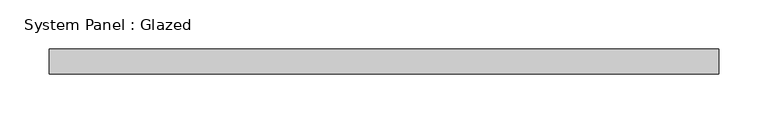
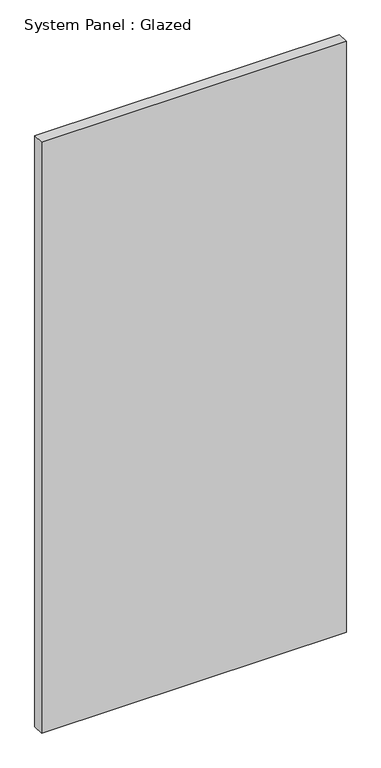
"""IFC4 building model written with IfcOpenShell, lengths in millimetres: plate geometry, System Panel : Glazed."""

from ifc_helpers import new_model, si_unit, origin, origin_with_axes, place, context, project, spatial, polyline, outline, extrude, source, transform, mapped, element, save


def system_panel_glazed_7e52d88a(model_context):
    return source(origin(), model_context, "Body", "SweptSolid", [
        extrude(outline(polyline([(338.6666667, 19.05), (-338.6666667, 19.05), (-338.6666667, 44.45), (338.6666667, 44.45), (338.6666667, 19.05)])), origin_with_axes(), (0.0, 0.0, 1.0), 1386.5761917),
    ])


if __name__ == "__main__":
    model = new_model("IFC4")
    model_context = context("Model", 3, world=origin())
    ifc_project = project(units=[si_unit("LENGTHUNIT", "METRE", prefix="MILLI")], contexts=[model_context])
    site = spatial("IfcSite", under=ifc_project)
    building = spatial("IfcBuilding", under=site)
    placement = place(None, origin())
    system_panel_glazed_shape = system_panel_glazed_7e52d88a(model_context)
    element("IfcPlate", 1, ObjectType="System Panel : Glazed", at=placement, inside=building, context=model_context, shape_type="MappedRepresentation", body=[
        mapped(system_panel_glazed_shape, transform((0.0, 0.0, 0.0), x_axis=(1.0, 0.0, 0.0), y_axis=(0.0, 1.0, 0.0), z_axis=(0.0, 0.0, 1.0))),
    ])
    save(model, "model.ifc")

# Revit data of these elements
# Type "System Panel : Glazed"
#   Construction Type Id = "GSP4R"
#   Analytic Construction = "1/8 in Pilkington single glazing"
#   Visual Light Transmittance = 0.9
#   Solar Heat Gain Coefficient = 0.86
#   Heat Transfer Coefficient (U) = 1.18115 BTU/(h·ft²·°F)
#   Define Thermal Properties by = 1
# Element 1 (IfcPlate, "System Panel : Glazed")
#   Materials on its faces: "Glass"
# Materials
#   "Glass": class "Glass", colour RGB 0 128 192, transparency 0.75, Description = "Soda Lime Glass", Cost = 0
